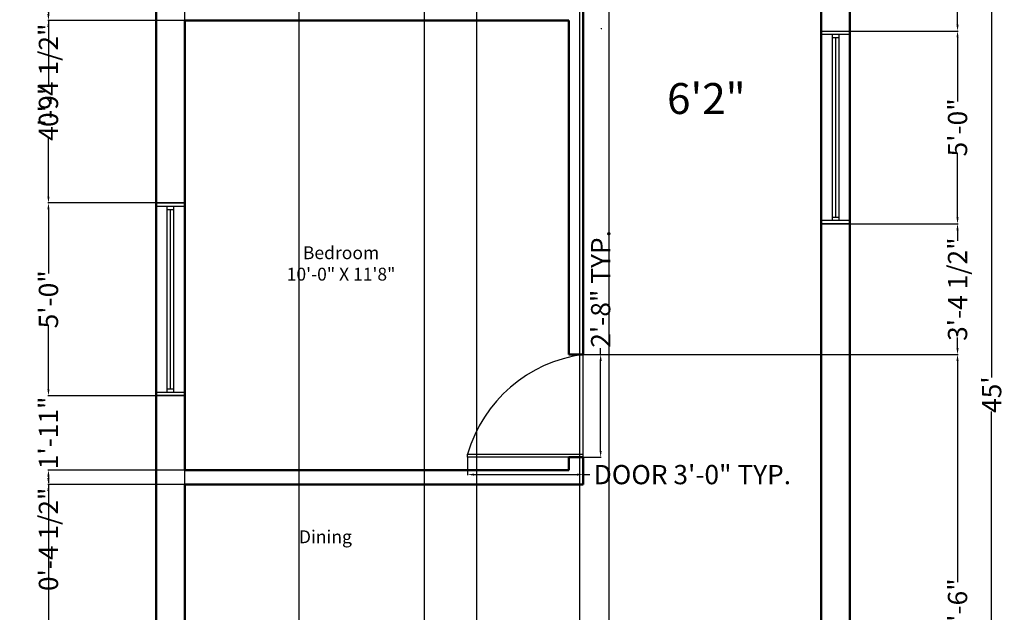
# Model space of a CAD drawing. Units: inches. Extents: x -34 to 296, y -84 to 618.
# Tile 2 of 3: x -11 to 296, y 238 to 423. Entities that reach past the tile are written whole.
import ezdxf

# ---------------------------------------------------------------- set-up
doc = ezdxf.new("R2010")
doc.units = ezdxf.units.IN
doc.header["$LTSCALE"] = 4
doc.header["$MEASUREMENT"] = 0
for name, color, linetype, lineweight in [('A-ANNO-DIMS', 2, 'Continuous', 18), ('A-AREA-IDEN', 3, 'Continuous', 18), ('A-DOOR', 4, 'Continuous', 25), ('A-GLAZ', 3, 'Continuous', 25), ('A-WALL', 7, 'Continuous', 50)]:
    doc.layers.add(name, color=color, linetype=linetype, lineweight=lineweight)
doc.styles.get("Standard").update_dxf_attribs({"font": 'arial.ttf'})
doc.dimstyles.get("Standard").update_dxf_attribs({"dimtxt": 6, "dimasz": 2, "dimexe": 0.18, "dimexo": 0.0625, "dimgap": 0.09, "dimtad": 0, "dimdec": 0, "dimzin": 0, "dimdsep": 46, "dimlunit": 4, "dimtxsty": 'Standard', "dimcen": 0.09, "dimadec": 0, "dimazin": 0, "dimtfac": 1, "dimtdec": 0, "dimtofl": 0, "dimtmove": 0, "dimatfit": 3, "dimfxl": 1, "dimtolj": 1, "dimtzin": 0, "dimarcsym": 0})

# ---------------------------------------------------------------- blocks, each defined once
blk = doc.blocks.new('*D2')
at = {"layer": 'A-ANNO-DIMS', "color": 0, "lineweight": -2, "transparency": 16777216}
for p, q in [((247.53, 576.03), (291.77, 576.03)), ((291.59, 574.03), (291.59, 311.33)), ((291.59, 38.03), (291.59, 300.73)), ((247.53, 36.03), (291.77, 36.03))]:
    blk.add_line(p, q, dxfattribs=at)
at = {"layer": 'A-ANNO-DIMS', "color": 0, "transparency": 16777216}
for points in [[(291.26, 574.03), (291.92, 574.03), (291.59, 576.03)], [(291.26, 38.03), (291.92, 38.03), (291.59, 36.03)]]:
    blk.add_solid(points, dxfattribs=at)
at = {"layer": 'Defpoints', "color": 0, "transparency": 16777216}
for p in [(247.47, 576.03), (247.47, 36.03), (291.59, 36.03)]:
    blk.add_point(p, dxfattribs=at)
at = {"layer": 'A-ANNO-DIMS', "color": 0, "transparency": 16777216, "insert": (291.59, 306.03), "char_height": 6, "attachment_point": 5, "rotation": 90}
blk.add_mtext("\\A1;45'", dxfattribs=at)
blk = doc.blocks.new('DOOR')
for p, q in [((177.71, 683.29), (177.71, 692.29)), ((177.71, 692.29), (237.71, 692.29)), ((178.71, 683.29), (178.71, 692.29)), ((236.71, 692.29), (236.71, 683.29)), ((237.71, 692.29), (237.71, 683.29)), ((178.71, 688.79), (236.71, 688.79)), ((178.71, 686.79), (236.71, 686.79)), ((179.71, 686.79), (179.71, 688.79)), ((179.71, 687.79), (235.71, 687.79)), ((235.71, 688.79), (235.71, 686.79)), ((237.71, 683.29), (177.71, 683.29))]:
    blk.add_line(p, q)
blk = doc.blocks.new('DOOR-900')
for p, q in [((36, 0), (36, 32)), ((0, 0), (0, 1)), ((0, 1), (36, 1)), ((36, 0), (0, 0))]:
    blk.add_line(p, q)
blk.add_arc((41.68, -11), 43.37, 97.5204, 163.9438)
blk = doc.blocks.new('*D10')
at = {"layer": 'A-ANNO-DIMS', "color": 0, "lineweight": -2, "transparency": 16777216}
for p, q in [((128.47, 286.47), (128.47, 280.95)), ((164.47, 286.47), (164.47, 280.95)), ((130.47, 281.13), (162.47, 281.13)), ((164.47, 281.13), (166.47, 281.13))]:
    blk.add_line(p, q, dxfattribs=at)
at = {"layer": 'A-ANNO-DIMS', "color": 0, "transparency": 16777216}
for points in [[(130.47, 281.47), (130.47, 280.8), (128.47, 281.13)], [(162.47, 281.47), (162.47, 280.8), (164.47, 281.13)]]:
    blk.add_solid(points, dxfattribs=at)
at = {"layer": 'Defpoints', "color": 0, "transparency": 16777216}
for p in [(128.47, 286.53), (164.47, 286.53), (164.47, 281.13)]:
    blk.add_point(p, dxfattribs=at)
at = {"layer": 'A-ANNO-DIMS', "color": 0, "transparency": 16777216, "insert": (198.43, 281.13), "char_height": 6, "attachment_point": 5}
blk.add_mtext('\\A1;DOOR 3\'-0" TYP.', dxfattribs=at)
blk = doc.blocks.new('*D11')
at = {"layer": 'A-ANNO-DIMS', "color": 0, "lineweight": -2, "transparency": 16777216}
for p, q in [((169.87, 318.53), (169.87, 320.53)), ((164.53, 318.53), (170.05, 318.53)), ((169.87, 288.53), (169.87, 316.53)), ((164.53, 286.53), (170.05, 286.53))]:
    blk.add_line(p, q, dxfattribs=at)
at = {"layer": 'A-ANNO-DIMS', "color": 0, "transparency": 16777216}
for points in [[(169.53, 316.53), (170.2, 316.53), (169.87, 318.53)], [(169.53, 288.53), (170.2, 288.53), (169.87, 286.53)]]:
    blk.add_solid(points, dxfattribs=at)
at = {"layer": 'Defpoints', "color": 0, "transparency": 16777216}
for p in [(164.47, 318.53), (169.87, 318.53), (164.47, 286.53)]:
    blk.add_point(p, dxfattribs=at)
at = {"layer": 'A-ANNO-DIMS', "color": 0, "transparency": 16777216, "insert": (169.87, 338.96), "char_height": 6, "attachment_point": 5, "rotation": 90}
blk.add_mtext('\\A1;2\'-8" TYP.', dxfattribs=at)
blk = doc.blocks.new('*D23')
at = {"layer": 'A-ANNO-DIMS', "color": 0, "lineweight": -2, "transparency": 16777216}
for p, q in [((40.4, 427.03), (-2.21, 427.03)), ((-2.03, 425.03), (-2.03, 424.53)), ((40.4, 422.53), (-2.21, 422.53)), ((-2.03, 422.53), (-2.03, 420.53))]:
    blk.add_line(p, q, dxfattribs=at)
at = {"layer": 'A-ANNO-DIMS', "color": 0, "transparency": 16777216}
for points in [[(-2.37, 425.03), (-1.7, 425.03), (-2.03, 427.03)], [(-2.37, 424.53), (-1.7, 424.53), (-2.03, 422.53)]]:
    blk.add_solid(points, dxfattribs=at)
at = {"layer": 'Defpoints', "color": 0, "transparency": 16777216}
for p in [(40.47, 427.03), (-2.03, 422.53), (40.47, 422.53)]:
    blk.add_point(p, dxfattribs=at)
at = {"layer": 'A-ANNO-DIMS', "color": 0, "transparency": 16777216, "insert": (-2.03, 405.48), "char_height": 6, "attachment_point": 5, "rotation": 90}
blk.add_mtext('\\A1;0\'-4 1/2"', dxfattribs=at)
blk = doc.blocks.new('*D24')
at = {"layer": 'A-ANNO-DIMS', "color": 0, "lineweight": -2, "transparency": 16777216}
for p, q in [((40.4, 422.53), (-2.21, 422.53)), ((-2.03, 420.53), (-2.03, 402.31)), ((-2.03, 367.71), (-2.03, 385.94)), ((40.4, 365.71), (-2.21, 365.71))]:
    blk.add_line(p, q, dxfattribs=at)
at = {"layer": 'A-ANNO-DIMS', "color": 0, "transparency": 16777216}
for points in [[(-2.37, 420.53), (-1.7, 420.53), (-2.03, 422.53)], [(-2.37, 367.71), (-1.7, 367.71), (-2.03, 365.71)]]:
    blk.add_solid(points, dxfattribs=at)
at = {"layer": 'Defpoints', "color": 0, "transparency": 16777216}
for p in [(40.47, 422.53), (-2.03, 365.71), (40.47, 365.71)]:
    blk.add_point(p, dxfattribs=at)
at = {"layer": 'A-ANNO-DIMS', "color": 0, "transparency": 16777216, "insert": (-2.03, 394.12), "char_height": 6, "attachment_point": 5, "rotation": 90}
blk.add_mtext('\\A1;4\'-9"', dxfattribs=at)
blk = doc.blocks.new('*D25')
at = {"layer": 'A-ANNO-DIMS', "color": 0, "lineweight": -2, "transparency": 16777216}
for p, q in [((40.4, 365.71), (-2.21, 365.71)), ((-2.03, 363.71), (-2.03, 343.78)), ((-2.03, 307.71), (-2.03, 327.65)), ((40.4, 305.71), (-2.21, 305.71))]:
    blk.add_line(p, q, dxfattribs=at)
at = {"layer": 'A-ANNO-DIMS', "color": 0, "transparency": 16777216}
for points in [[(-2.37, 363.71), (-1.7, 363.71), (-2.03, 365.71)], [(-2.37, 307.71), (-1.7, 307.71), (-2.03, 305.71)]]:
    blk.add_solid(points, dxfattribs=at)
at = {"layer": 'Defpoints', "color": 0, "transparency": 16777216}
for p in [(40.47, 365.71), (-2.03, 305.71), (40.47, 305.71)]:
    blk.add_point(p, dxfattribs=at)
at = {"layer": 'A-ANNO-DIMS', "color": 0, "transparency": 16777216, "insert": (-2.03, 335.71), "char_height": 6, "attachment_point": 5, "rotation": 90}
blk.add_mtext('\\A1;5\'-0"', dxfattribs=at)
blk = doc.blocks.new('*D26')
at = {"layer": 'A-ANNO-DIMS', "color": 0, "lineweight": -2, "transparency": 16777216}
for p, q in [((-2.03, 307.71), (-2.03, 309.71)), ((40.4, 305.71), (-2.21, 305.71)), ((40.4, 282.53), (-2.21, 282.53)), ((-2.03, 280.53), (-2.03, 278.53))]:
    blk.add_line(p, q, dxfattribs=at)
at = {"layer": 'A-ANNO-DIMS', "color": 0, "transparency": 16777216}
for points in [[(-2.37, 307.71), (-1.7, 307.71), (-2.03, 305.71)], [(-2.37, 280.53), (-1.7, 280.53), (-2.03, 282.53)]]:
    blk.add_solid(points, dxfattribs=at)
at = {"layer": 'Defpoints', "color": 0, "transparency": 16777216}
for p in [(40.47, 305.71), (-2.03, 282.53), (40.47, 282.53)]:
    blk.add_point(p, dxfattribs=at)
at = {"layer": 'A-ANNO-DIMS', "color": 0, "transparency": 16777216, "insert": (-2.03, 294.12), "char_height": 6, "attachment_point": 5, "rotation": 90}
blk.add_mtext('\\A1;1\'-11"', dxfattribs=at)
blk = doc.blocks.new('*D27')
at = {"layer": 'A-ANNO-DIMS', "color": 0, "lineweight": -2, "transparency": 16777216}
for p, q in [((40.4, 282.53), (-2.21, 282.53)), ((-2.03, 280.53), (-2.03, 280.03)), ((40.4, 278.03), (-2.21, 278.03)), ((-2.03, 278.03), (-2.03, 276.03))]:
    blk.add_line(p, q, dxfattribs=at)
at = {"layer": 'A-ANNO-DIMS', "color": 0, "transparency": 16777216}
for points in [[(-2.37, 280.53), (-1.7, 280.53), (-2.03, 282.53)], [(-2.37, 280.03), (-1.7, 280.03), (-2.03, 278.03)]]:
    blk.add_solid(points, dxfattribs=at)
at = {"layer": 'Defpoints', "color": 0, "transparency": 16777216}
for p in [(40.47, 282.53), (-2.03, 278.03), (40.47, 278.03)]:
    blk.add_point(p, dxfattribs=at)
at = {"layer": 'A-ANNO-DIMS', "color": 0, "transparency": 16777216, "insert": (-2.03, 260.98), "char_height": 6, "attachment_point": 5, "rotation": 90}
blk.add_mtext('\\A1;0\'-4 1/2"', dxfattribs=at)
blk = doc.blocks.new('*D28')
at = {"layer": 'A-ANNO-DIMS', "color": 0, "lineweight": -2, "transparency": 16777216}
for p, q in [((40.4, 278.03), (-2.21, 278.03)), ((-2.03, 276.03), (-2.03, 220.89)), ((-2.03, 131.53), (-2.03, 186.68)), ((40.4, 129.53), (-2.21, 129.53))]:
    blk.add_line(p, q, dxfattribs=at)
at = {"layer": 'A-ANNO-DIMS', "color": 0, "transparency": 16777216}
for points in [[(-2.37, 276.03), (-1.7, 276.03), (-2.03, 278.03)], [(-2.37, 131.53), (-1.7, 131.53), (-2.03, 129.53)]]:
    blk.add_solid(points, dxfattribs=at)
at = {"layer": 'Defpoints', "color": 0, "transparency": 16777216}
for p in [(40.47, 278.03), (-2.03, 129.53), (40.47, 129.53)]:
    blk.add_point(p, dxfattribs=at)
at = {"layer": 'A-ANNO-DIMS', "color": 0, "transparency": 16777216, "insert": (-2.03, 203.78), "char_height": 6, "attachment_point": 5, "rotation": 90}
blk.add_mtext('\\A1;12\'-4 1/2"', dxfattribs=at)
blk = doc.blocks.new('*D36')
at = {"layer": 'A-ANNO-DIMS', "color": 0, "lineweight": -2, "transparency": 16777216}
for p, q in [((238.53, 468.03), (281.15, 468.03)), ((280.97, 466.03), (280.97, 451.82)), ((280.97, 421.24), (280.97, 435.45)), ((238.53, 419.24), (281.15, 419.24))]:
    blk.add_line(p, q, dxfattribs=at)
at = {"layer": 'A-ANNO-DIMS', "color": 0, "transparency": 16777216}
for points in [[(280.63, 466.03), (281.3, 466.03), (280.97, 468.03)], [(280.63, 421.24), (281.3, 421.24), (280.97, 419.24)]]:
    blk.add_solid(points, dxfattribs=at)
at = {"layer": 'Defpoints', "color": 0, "transparency": 16777216}
for p in [(238.47, 468.03), (238.47, 419.24), (280.97, 419.24)]:
    blk.add_point(p, dxfattribs=at)
at = {"layer": 'A-ANNO-DIMS', "color": 0, "transparency": 16777216, "insert": (280.97, 443.63), "char_height": 6, "attachment_point": 5, "rotation": 90}
blk.add_mtext('\\A1;4\'-1"', dxfattribs=at)
blk = doc.blocks.new('*D37')
at = {"layer": 'A-ANNO-DIMS', "color": 0, "lineweight": -2, "transparency": 16777216}
for p, q in [((238.53, 419.24), (281.15, 419.24)), ((280.97, 417.24), (280.97, 397.3)), ((280.97, 361.24), (280.97, 381.17)), ((238.53, 359.24), (281.15, 359.24))]:
    blk.add_line(p, q, dxfattribs=at)
at = {"layer": 'A-ANNO-DIMS', "color": 0, "transparency": 16777216}
for points in [[(280.63, 417.24), (281.3, 417.24), (280.97, 419.24)], [(280.63, 361.24), (281.3, 361.24), (280.97, 359.24)]]:
    blk.add_solid(points, dxfattribs=at)
at = {"layer": 'Defpoints', "color": 0, "transparency": 16777216}
for p in [(238.47, 419.24), (238.47, 359.24), (280.97, 359.24)]:
    blk.add_point(p, dxfattribs=at)
at = {"layer": 'A-ANNO-DIMS', "color": 0, "transparency": 16777216, "insert": (280.97, 389.24), "char_height": 6, "attachment_point": 5, "rotation": 90}
blk.add_mtext('\\A1;5\'-0"', dxfattribs=at)
blk = doc.blocks.new('*D38')
at = {"layer": 'A-ANNO-DIMS', "color": 0, "lineweight": -2, "transparency": 16777216}
for p, q in [((238.53, 359.24), (281.15, 359.24)), ((280.97, 357.24), (280.97, 353.94)), ((280.97, 320.53), (280.97, 323.83)), ((164.53, 318.53), (281.15, 318.53))]:
    blk.add_line(p, q, dxfattribs=at)
at = {"layer": 'A-ANNO-DIMS', "color": 0, "transparency": 16777216}
for points in [[(280.63, 357.24), (281.3, 357.24), (280.97, 359.24)], [(280.63, 320.53), (281.3, 320.53), (280.97, 318.53)]]:
    blk.add_solid(points, dxfattribs=at)
at = {"layer": 'Defpoints', "color": 0, "transparency": 16777216}
for p in [(238.47, 359.24), (164.47, 318.53), (280.97, 318.53)]:
    blk.add_point(p, dxfattribs=at)
at = {"layer": 'A-ANNO-DIMS', "color": 0, "transparency": 16777216, "insert": (280.97, 338.88), "char_height": 6, "attachment_point": 5, "rotation": 90}
blk.add_mtext('\\A1;3\'-4 1/2"', dxfattribs=at)
blk = doc.blocks.new('*D39')
at = {"layer": 'A-ANNO-DIMS', "color": 0, "lineweight": -2, "transparency": 16777216}
for p, q in [((164.53, 318.53), (281.15, 318.53)), ((280.97, 316.53), (280.97, 247.63)), ((280.97, 158.5), (280.97, 227.4)), ((238.53, 156.5), (281.15, 156.5))]:
    blk.add_line(p, q, dxfattribs=at)
at = {"layer": 'A-ANNO-DIMS', "color": 0, "transparency": 16777216}
for points in [[(280.63, 316.53), (281.3, 316.53), (280.97, 318.53)], [(280.63, 158.5), (281.3, 158.5), (280.97, 156.5)]]:
    blk.add_solid(points, dxfattribs=at)
at = {"layer": 'Defpoints', "color": 0, "transparency": 16777216}
for p in [(164.47, 318.53), (238.47, 156.5), (280.97, 156.5)]:
    blk.add_point(p, dxfattribs=at)
at = {"layer": 'A-ANNO-DIMS', "color": 0, "transparency": 16777216, "insert": (280.97, 237.51), "char_height": 6, "attachment_point": 5, "rotation": 90}
blk.add_mtext('\\A1;13\'-6"', dxfattribs=at)
blk = doc.blocks.new('*D51')
at = {"layer": 'A-ANNO-DIMS', "color": 0, "lineweight": -2, "transparency": 16777216}
for p, q in [((38.47, 609.53), (36.47, 609.53)), ((40.47, 129.6), (40.47, 609.71)), ((76.01, 129.6), (76.01, 609.71)), ((78.01, 609.53), (80.01, 609.53))]:
    blk.add_line(p, q, dxfattribs=at)
at = {"layer": 'A-ANNO-DIMS', "color": 0, "transparency": 16777216}
for points in [[(38.47, 609.87), (38.47, 609.2), (40.47, 609.53)], [(78.01, 609.87), (78.01, 609.2), (76.01, 609.53)]]:
    blk.add_solid(points, dxfattribs=at)
at = {"layer": 'Defpoints', "color": 0, "transparency": 16777216}
for p in [(76.01, 609.53), (40.47, 129.53), (76.01, 129.53)]:
    blk.add_point(p, dxfattribs=at)
at = {"layer": 'A-ANNO-DIMS', "color": 0, "transparency": 16777216, "insert": (58.24, 609.53), "char_height": 6, "attachment_point": 5}
blk.add_mtext('\\A1;2\'-11 1/2"', dxfattribs=at)
blk = doc.blocks.new('*D52')
at = {"layer": 'A-ANNO-DIMS', "color": 0, "lineweight": -2, "transparency": 16777216}
for p, q in [((76.01, 129.6), (76.01, 609.71)), ((78.01, 609.53), (87.45, 609.53)), ((113.01, 609.53), (103.57, 609.53)), ((115.01, 129.6), (115.01, 609.71))]:
    blk.add_line(p, q, dxfattribs=at)
at = {"layer": 'A-ANNO-DIMS', "color": 0, "transparency": 16777216}
for points in [[(78.01, 609.87), (78.01, 609.2), (76.01, 609.53)], [(113.01, 609.87), (113.01, 609.2), (115.01, 609.53)]]:
    blk.add_solid(points, dxfattribs=at)
at = {"layer": 'Defpoints', "color": 0, "transparency": 16777216}
for p in [(115.01, 609.53), (76.01, 129.53), (115.01, 129.53)]:
    blk.add_point(p, dxfattribs=at)
at = {"layer": 'A-ANNO-DIMS', "color": 0, "transparency": 16777216, "insert": (95.51, 609.53), "char_height": 6, "attachment_point": 5}
blk.add_mtext('\\A1;3\'-3"', dxfattribs=at)
blk = doc.blocks.new('*D53')
at = {"layer": 'A-ANNO-DIMS', "color": 0, "lineweight": -2, "transparency": 16777216}
for p, q in [((115.01, 129.6), (115.01, 609.71)), ((117.01, 609.53), (129.36, 609.53)), ((131.36, 129.6), (131.36, 609.71)), ((131.36, 609.53), (133.36, 609.53))]:
    blk.add_line(p, q, dxfattribs=at)
at = {"layer": 'A-ANNO-DIMS', "color": 0, "transparency": 16777216}
for points in [[(117.01, 609.87), (117.01, 609.2), (115.01, 609.53)], [(129.36, 609.87), (129.36, 609.2), (131.36, 609.53)]]:
    blk.add_solid(points, dxfattribs=at)
at = {"layer": 'Defpoints', "color": 0, "transparency": 16777216}
for p in [(131.36, 609.53), (115.01, 129.53), (131.36, 129.53)]:
    blk.add_point(p, dxfattribs=at)
at = {"layer": 'A-ANNO-DIMS', "color": 0, "transparency": 16777216, "insert": (148.13, 609.53), "char_height": 6, "attachment_point": 5}
blk.add_mtext('\\A1;1\'-4 1/2"', dxfattribs=at)
blk = doc.blocks.new('*D54')
at = {"layer": 'A-ANNO-DIMS', "color": 0, "lineweight": -2, "transparency": 16777216}
for p, q in [((131.36, 129.6), (131.36, 609.71)), ((133.36, 609.53), (139.24, 609.53)), ((161.36, 609.53), (155.48, 609.53)), ((163.36, 129.6), (163.36, 609.71))]:
    blk.add_line(p, q, dxfattribs=at)
at = {"layer": 'A-ANNO-DIMS', "color": 0, "transparency": 16777216}
for points in [[(133.36, 609.87), (133.36, 609.2), (131.36, 609.53)], [(161.36, 609.87), (161.36, 609.2), (163.36, 609.53)]]:
    blk.add_solid(points, dxfattribs=at)
at = {"layer": 'Defpoints', "color": 0, "transparency": 16777216}
for p in [(163.36, 609.53), (131.36, 129.53), (163.36, 129.53)]:
    blk.add_point(p, dxfattribs=at)
at = {"layer": 'A-ANNO-DIMS', "color": 0, "transparency": 16777216, "insert": (147.36, 609.53), "char_height": 6, "attachment_point": 5}
blk.add_mtext('\\A1;2\'-8"', dxfattribs=at)
blk = doc.blocks.new('*D55')
at = {"layer": 'A-ANNO-DIMS', "color": 0, "lineweight": -2, "transparency": 16777216}
for p, q in [((163.36, 129.6), (163.36, 609.71)), ((165.36, 609.53), (170.47, 609.53)), ((172.47, 129.6), (172.47, 609.71)), ((172.47, 609.53), (174.47, 609.53))]:
    blk.add_line(p, q, dxfattribs=at)
at = {"layer": 'A-ANNO-DIMS', "color": 0, "transparency": 16777216}
for points in [[(165.36, 609.87), (165.36, 609.2), (163.36, 609.53)], [(170.47, 609.87), (170.47, 609.2), (172.47, 609.53)]]:
    blk.add_solid(points, dxfattribs=at)
at = {"layer": 'Defpoints', "color": 0, "transparency": 16777216}
for p in [(172.47, 609.53), (163.36, 129.53), (172.47, 129.53)]:
    blk.add_point(p, dxfattribs=at)
at = {"layer": 'A-ANNO-DIMS', "color": 0, "transparency": 16777216, "insert": (182.53, 609.53), "char_height": 6, "attachment_point": 5}
blk.add_mtext('\\A1;0\'-9"', dxfattribs=at)
blk = doc.blocks.new('*D59')
at = {"layer": 'A-ANNO-DIMS', "color": 0, "lineweight": -2, "transparency": 16777216}
for p, q in [((139.23, 455.93), (140.54, 454.42)), ((170.05, 420.04), (170.23, 420.04)), ((170.14, 419.95), (170.14, 420.13))]:
    blk.add_line(p, q, dxfattribs=at)
at = {"layer": 'A-ANNO-DIMS', "color": 0, "transparency": 16777216}
blk.add_solid([(140.79, 454.63), (140.29, 454.2), (141.84, 452.9)], dxfattribs=at)
at = {"layer": 'Defpoints', "color": 0, "transparency": 16777216}
for p in [(141.84, 452.9), (170.14, 420.04)]:
    blk.add_point(p, dxfattribs=at)
at = {"layer": 'A-ANNO-DIMS', "color": 0, "transparency": 16777216, "insert": (123.33, 474.4), "char_height": 6, "attachment_point": 5, "rotation": 310.7319}
blk.add_mtext('\\A1;3X R3\'-7 1/2"', dxfattribs=at)

msp = doc.modelspace()

# ---------------------------------------------------------------- linework, layer by layer
at = {"layer": 'A-WALL'}
for p, q in [((31.47, 36.03), (31.47, 576.03)), ((247.47, 576.03), (247.47, 36.03)), ((238.47, 468.03), (238.47, 45.03)), ((164.47, 431.03), (164.47, 318.53)), ((40.47, 422.53), (159.97, 422.53)), ((40.47, 282.53), (40.47, 422.53)), ((159.97, 422.53), (159.97, 318.53)), ((159.97, 318.53), (164.47, 318.53)), ((159.97, 286.53), (164.47, 286.53)), ((159.97, 286.53), (159.97, 282.53)), ((164.47, 286.53), (164.47, 278.03)), ((40.47, 282.53), (159.97, 282.53)), ((40.47, 278.03), (164.47, 278.03)), ((40.47, 129.53), (40.47, 278.03))]:
    msp.add_line(p, q, dxfattribs=at)

# ---------------------------------------------------------------- block references
at = {"layer": 'A-DOOR'}
msp.add_blockref('DOOR-900', (128.47, 286.53), dxfattribs=at)
at = {"layer": 'A-GLAZ'}
for p, rotation in [((-444.82, 596.94), 270), ((723.75, 128.01), 90)]:
    msp.add_blockref('DOOR', p, dxfattribs=dict(at, rotation=rotation))

# ---------------------------------------------------------------- texts
at = {"layer": 'A-AREA-IDEN', "attachment_point": 1}
for s, width, gutter_width, insert, char_height in [('\\pxqc;6\'2"', 104.4689, 48.17, (150.54, 403.05), 9.633), ('\\pxqc;Bedroom\\P10\'-0" X 11\'8"', 62.1792, 20, (57.97, 352.21), 4), ('\\pxqc;Dining', 71.969, 20, (48.21, 263.78), 4)]:
    msp.add_mtext_dynamic_manual_height_columns(s, width=width, gutter_width=gutter_width, heights=[0], dxfattribs=dict(at, insert=insert, char_height=char_height))

# ---------------------------------------------------------------- dimensions: what is measured, and where the dimension line sits
at = {"layer": 'A-ANNO-DIMS'}
for base, p1, p2, picture, middle in [((76.01, 609.53), (40.47, 129.53), (76.01, 129.53), '*D51', (58.24, 609.53)), ((131.3602, 609.5325), (115.0111, 129.5325), (131.3602, 129.5325), '*D53', (148.133, 609.5325)), ((115.01, 609.53), (76.01, 129.53), (115.01, 129.53), '*D52', (95.51, 609.53)), ((163.36, 609.53), (131.36, 129.53), (163.36, 129.53), '*D54', (147.36, 609.53)), ((172.47, 609.53), (163.36, 129.53), (172.47, 129.53), '*D55', (182.53, 609.53))]:
    dim = msp.add_linear_dim(base=base, p1=p1, p2=p2, dimstyle='Standard', override={"dimdec": 1, "dimlfac": 1, "dimrnd": 0, "dimzin": 1, "dimdsep": 46, "dimlunit": 4, "dimfrac": 2}, dxfattribs=at)
    dim.commit()
    dim.dimension.update_dxf_attribs({"geometry": picture, "text_midpoint": middle})
for base, p1, p2, override, picture, middle in [((291.59, 36.03), (247.47, 576.03), (247.47, 36.03), {"dimclrd": 0, "dimclre": 0, "dimclrt": 0}, '*D2', (291.59, 306.03)), ((280.97, 419.24), (238.47, 468.03), (238.47, 419.24), {"dimdec": 1, "dimlfac": 1, "dimrnd": 0, "dimzin": 1, "dimdsep": 46, "dimlunit": 4, "dimfrac": 2}, '*D36', (280.97, 443.63)), ((-2.03, 422.53), (40.47, 427.03), (40.47, 422.53), {"dimdec": 1, "dimlfac": 1, "dimrnd": 0, "dimzin": 1, "dimdsep": 46, "dimlunit": 4, "dimfrac": 2}, '*D23', (-2.03, 405.48)), ((-2.03, 365.71), (40.47, 422.53), (40.47, 365.71), {"dimdec": 1, "dimlfac": 1, "dimrnd": 0, "dimzin": 1, "dimdsep": 46, "dimlunit": 4, "dimfrac": 2}, '*D24', (-2.03, 394.12)), ((280.97, 359.24), (238.47, 419.24), (238.47, 359.24), {"dimdec": 1, "dimlfac": 1, "dimrnd": 0, "dimzin": 1, "dimdsep": 46, "dimlunit": 4, "dimfrac": 2}, '*D37', (280.97, 389.24)), ((-2.03, 305.71), (40.47, 365.71), (40.47, 305.71), {"dimdec": 1, "dimlfac": 1, "dimrnd": 0, "dimzin": 1, "dimdsep": 46, "dimlunit": 4, "dimfrac": 2}, '*D25', (-2.03, 335.71)), ((280.97, 318.53), (238.47, 359.24), (164.47, 318.53), {"dimdec": 1, "dimlfac": 1, "dimrnd": 0, "dimzin": 1, "dimdsep": 46, "dimlunit": 4, "dimfrac": 2}, '*D38', (280.97, 338.88)), ((280.97, 156.5), (164.47, 318.53), (238.47, 156.5), {"dimdec": 1, "dimlfac": 1, "dimrnd": 0, "dimzin": 1, "dimdsep": 46, "dimlunit": 4, "dimfrac": 2}, '*D39', (280.97, 237.51)), ((-2.03, 282.53), (40.47, 305.71), (40.47, 282.53), {"dimdec": 1, "dimlfac": 1, "dimrnd": 0, "dimzin": 1, "dimdsep": 46, "dimlunit": 4, "dimfrac": 2}, '*D26', (-2.03, 294.12)), ((-2.03, 278.03), (40.47, 282.53), (40.47, 278.03), {"dimdec": 1, "dimlfac": 1, "dimrnd": 0, "dimzin": 1, "dimdsep": 46, "dimlunit": 4, "dimfrac": 2}, '*D27', (-2.03, 260.98)), ((-2.03, 129.53), (40.47, 278.03), (40.47, 129.53), {"dimdec": 1, "dimlfac": 1, "dimrnd": 0, "dimzin": 1, "dimdsep": 46, "dimlunit": 4, "dimfrac": 2}, '*D28', (-2.03, 203.78))]:
    dim = msp.add_linear_dim(base=base, p1=p1, p2=p2, angle=90, dimstyle='Standard', override=override, dxfattribs=at)
    dim.commit()
    dim.dimension.update_dxf_attribs({"geometry": picture, "text_midpoint": middle})
dim = msp.add_radius_dim(center=(170.14, 420.04), mpoint=(141.84, 452.9), text='3X <>', dimstyle='Standard', override={"dimdec": 1, "dimlfac": 1, "dimrnd": 0, "dimzin": 1, "dimdsep": 46, "dimlunit": 4, "dimfrac": 2}, dxfattribs=at)
dim.commit()
dim.dimension.update_dxf_attribs({"geometry": '*D59', "text_midpoint": (123.33, 474.4)})
dim = msp.add_linear_dim(base=(169.87, 318.53), p1=(164.47, 286.53), p2=(164.47, 318.53), angle=90, text='<> TYP.', dimstyle='Standard', override={"dimdec": 1, "dimrnd": 0, "dimzin": 1, "dimlunit": 4, "dimfrac": 2}, dxfattribs=at)
dim.commit()
dim.dimension.update_dxf_attribs({"geometry": '*D11', "text_midpoint": (169.87, 338.96)})
dim = msp.add_linear_dim(base=(164.47, 281.13), p1=(128.47, 286.53), p2=(164.47, 286.53), text='DOOR <> TYP.', dimstyle='Standard', override={"dimdec": 1, "dimrnd": 0, "dimzin": 1, "dimlunit": 4, "dimfrac": 2}, dxfattribs=at)
dim.commit()
dim.dimension.update_dxf_attribs({"geometry": '*D10', "text_midpoint": (198.43, 281.13)})

doc.saveas('drawing.dxf')
